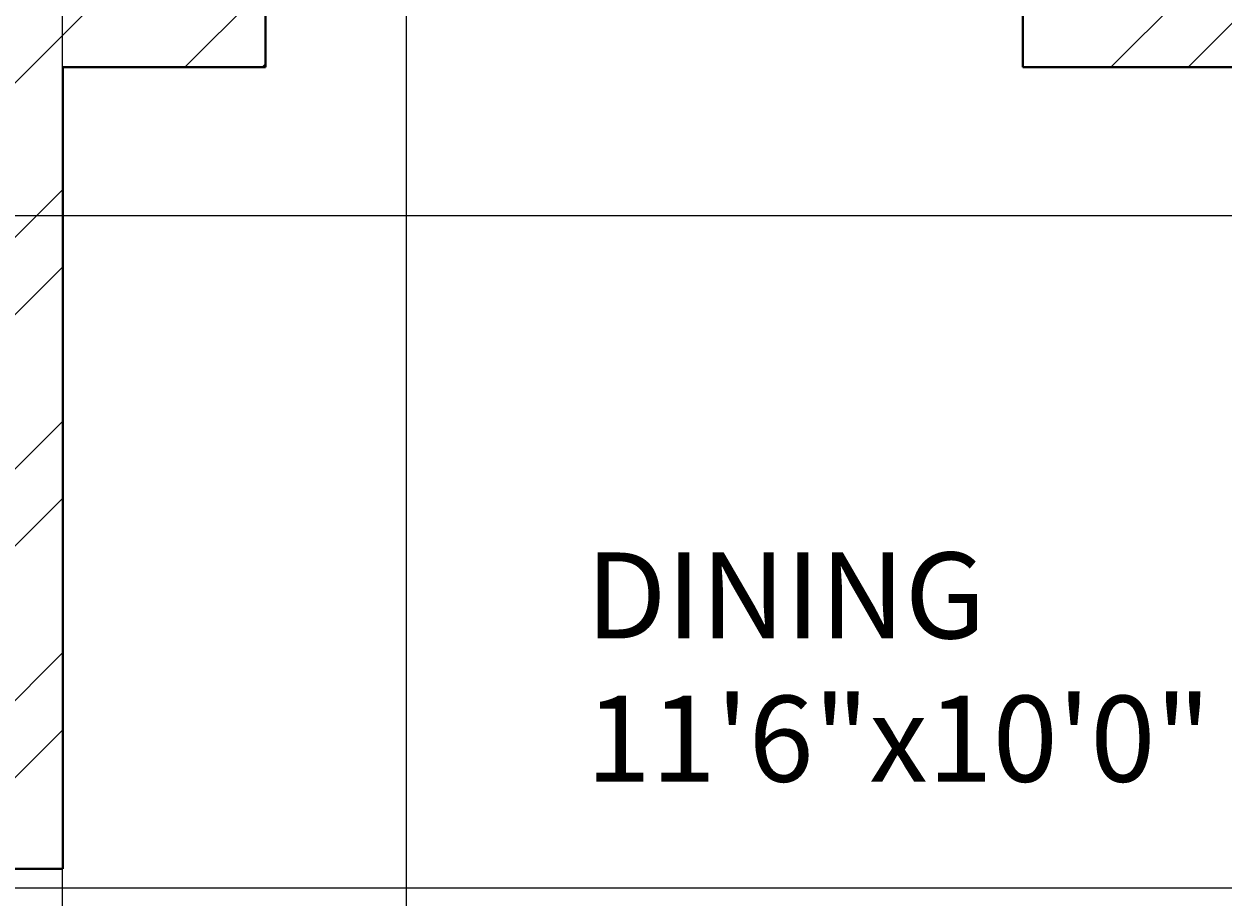
# Model space of a CAD drawing. Units: inches. Extents: x 1601 to 2297, y 1496 to 2631.
# Tile 53 of 57: x 2033 to 2103, y 2371 to 2422. Entities that reach past the tile are written whole.
import ezdxf

# ---------------------------------------------------------------- set-up
doc = ezdxf.new("R2010")
doc.units = ezdxf.units.IN
for name, color, linetype, lineweight in [('A-ANNO-DIMS', 2, 'Continuous', 18), ('A-AREA-IDEN', 7, 'Continuous', 18), ('A-WALL', 7, 'Continuous', 40), ('A-WALL-PATT', 215, 'Continuous', 13)]:
    doc.layers.add(name, color=color, linetype=linetype, lineweight=lineweight)
doc.styles.get("Standard").update_dxf_attribs({"font": 'arial.ttf'})
doc.dimstyles.get("Standard").update_dxf_attribs({"dimtxt": 0.18, "dimasz": 0.18, "dimexe": 0.18, "dimexo": 0.0625, "dimgap": 0.09, "dimtad": 0, "dimtih": 1, "dimtoh": 1, "dimdec": 4, "dimzin": 0, "dimdsep": 46, "dimtxsty": 'Standard', "dimcen": 0.09, "dimadec": 0, "dimazin": 0, "dimtfac": 1, "dimtdec": 4, "dimtofl": 0, "dimtmove": 0, "dimatfit": 3, "dimfxl": 1, "dimtolj": 1, "dimtzin": 0, "dimarcsym": 0})

# ---------------------------------------------------------------- blocks, each defined once
blk = doc.blocks.new('*D40')
at = {"layer": 'A-ANNO-DIMS', "color": 0, "lineweight": -2, "transparency": 16777216}
for p, q in [((2035.537, 1986.388), (2035.537, 2581.055)), ((2035.717, 2580.875), (2045.079, 2580.875)), ((2055.371, 2580.875), (2046.009, 2580.875)), ((2055.551, 1986.388), (2055.551, 2581.055))]:
    blk.add_line(p, q, dxfattribs=at)
at = {"layer": 'A-ANNO-DIMS', "color": 0, "transparency": 16777216}
for points in [[(2035.717, 2580.905), (2035.717, 2580.845), (2035.537, 2580.875)], [(2055.371, 2580.905), (2055.371, 2580.845), (2055.551, 2580.875)]]:
    blk.add_solid(points, dxfattribs=at)
at = {"layer": 'Defpoints', "color": 0, "transparency": 16777216}
for p in [(2055.551, 2580.875), (2035.537, 1986.325), (2055.551, 1986.325)]:
    blk.add_point(p, dxfattribs=at)
at = {"layer": 'A-ANNO-DIMS', "color": 0, "transparency": 16777216, "insert": (2045.544, 2580.875), "char_height": 0.18, "attachment_point": 5}
blk.add_mtext('\\A1;20.014', dxfattribs=at)
blk = doc.blocks.new('*D51')
at = {"layer": 'A-ANNO-DIMS', "color": 0, "lineweight": -2, "transparency": 16777216}
for p, q in [((1912.152, 2411.194), (2279.267, 2411.194)), ((2279.087, 2411.014), (2279.087, 2391.827)), ((2279.087, 2372.275), (2279.087, 2391.463)), ((1912.152, 2372.095), (2279.267, 2372.095))]:
    blk.add_line(p, q, dxfattribs=at)
at = {"layer": 'A-ANNO-DIMS', "color": 0, "transparency": 16777216}
for points in [[(2279.057, 2411.014), (2279.117, 2411.014), (2279.087, 2411.194)], [(2279.057, 2372.275), (2279.117, 2372.275), (2279.087, 2372.095)]]:
    blk.add_solid(points, dxfattribs=at)
at = {"layer": 'Defpoints', "color": 0, "transparency": 16777216}
for p in [(1912.09, 2411.194), (2279.087, 2411.194), (1912.09, 2372.095)]:
    blk.add_point(p, dxfattribs=at)
at = {"layer": 'A-ANNO-DIMS', "color": 0, "transparency": 16777216, "insert": (2279.087, 2391.645), "char_height": 0.18, "attachment_point": 5}
blk.add_mtext('\\A1;39.1', dxfattribs=at)

msp = doc.modelspace()

# ---------------------------------------------------------------- hatches: boundary and pattern name
at = {"layer": 'A-WALL-PATT'}
h = msp.add_hatch(dxfattribs=at)
h.set_pattern_fill('ANSI32', color=256)
h.paths.add_polyline_path([(1842.0336, 2528.0767), (1842.0336, 2532.3254), (1686.0373, 2532.3254), (1686.0373, 2492.9493), (1695.0373, 2492.9493), (1695.0373, 2523.3254), (1827.0373, 2523.3254), (1827.0373, 2416.8254), (1834.6225, 2416.8254), (1834.6225, 2419.0754), (1834.6225, 2421.3254), (1831.5373, 2421.3254), (1831.5373, 2523.3254), (1842.0336, 2523.3254)])
h.paths.add_polyline_path([(1695.0373, 2432.9493), (1686.0373, 2432.9493), (1686.0373, 2325.989), (1695.0373, 2325.989), (1695.0373, 2347.8254), (1827.0373, 2347.8254), (1827.0373, 2287.8254), (1823.2991, 2287.8254), (1823.2991, 2283.3254), (1847.9422, 2283.3254), (1847.9422, 2285.5754), (1847.9422, 2287.8254), (1831.5373, 2287.8254), (1831.5373, 2347.8254), (1846.9946, 2347.8254), (1846.9946, 2350.0754), (1846.9946, 2352.3254), (1695.0373, 2352.3254)])
h.paths.add_polyline_path([(1807.1169, 1573.5395), (2055.0405, 1573.5395), (2055.0405, 1610.6322), (1807.1169, 1610.6322)], flags=9)
h.paths.add_polyline_path([(1841.1631, 1712.7967), (1870.3957, 1712.7967), (1870.3957, 1731.454), (1841.1631, 1731.454)], flags=9)
h.paths.add_polyline_path([(2144.3862, 1772.185), (2191.0233, 1772.185), (2191.0233, 1790.8423), (2144.3862, 1790.8423)], flags=9)
h.paths.add_polyline_path([(2143.0128, 1827.3312), (2177.9958, 1827.3312), (2177.9958, 1845.9886), (2143.0128, 1845.9886)], flags=9)
h.paths.add_polyline_path([(2041.2439, 1833.5691), (2070.8516, 1833.5691), (2070.8516, 1852.2264), (2041.2439, 1852.2264)], flags=9)
h.paths.add_polyline_path([(2097.2791, 1947.0598), (2134.2061, 1947.0598), (2134.2061, 1965.7171), (2097.2791, 1965.7171)], flags=9)
h.paths.add_polyline_path([(2214.995, 1904.3124), (2214.995, 1942.2899), (2196.3376, 1942.2899), (2196.3376, 1904.3124)], flags=9)
h.paths.add_polyline_path([(2186.6284, 2043.8031), (2219.7935, 2043.8031), (2219.7935, 2062.4605), (2186.6284, 2062.4605)], flags=9)
h.paths.add_polyline_path([(2064.0877, 2031.616), (2097.4949, 2031.616), (2097.4949, 2050.2734), (2064.0877, 2050.2734)], flags=9)
h.paths.add_polyline_path([(1973.1349, 1986.0688), (2008.4009, 1986.0688), (2008.4009, 2004.7261), (1973.1349, 2004.7261)], flags=9)
h.paths.add_polyline_path([(1976.3676, 2106.9635), (2005.7469, 2106.9635), (2005.7469, 2125.6209), (1976.3676, 2125.6209)], flags=9)
h.paths.add_polyline_path([(1991.7852, 2180.4863), (2027.0513, 2180.4863), (2027.0513, 2199.1437), (1991.7852, 2199.1437)], flags=9)
h.paths.add_polyline_path([(2106.1801, 2187.9359), (2152.2101, 2187.9359), (2152.2101, 2206.5932), (2106.1801, 2206.5932)], flags=9)
h.paths.add_polyline_path([(2148.6686, 2262.2542), (2182.318, 2262.2542), (2182.318, 2280.9115), (2148.6686, 2280.9115)], flags=9)
h.paths.add_polyline_path([(2041.6327, 2252.8147), (2071.2405, 2252.8147), (2071.2405, 2271.4721), (2041.6327, 2271.4721)], flags=9)
h.paths.add_polyline_path([(2063.9734, 2375.4265), (2100.9004, 2375.4265), (2100.9004, 2394.0839), (2063.9734, 2394.0839)], flags=9)
h.paths.add_polyline_path([(2216.4955, 2330.9748), (2216.4955, 2370.2654), (2197.8381, 2370.2654), (2197.8381, 2330.9748)], flags=9)
h.paths.add_polyline_path([(2179.1416, 2485.8687), (2212.3067, 2485.8687), (2212.3067, 2504.5261), (2179.1416, 2504.5261)], flags=9)
h.paths.add_polyline_path([(2078.7442, 2471.1516), (2112.1514, 2471.1516), (2112.1514, 2489.809), (2078.7442, 2489.809)], flags=9)
h.paths.add_polyline_path([(1915.9631, 2329.4668), (1952.8902, 2329.4668), (1952.8902, 2348.1241), (1915.9631, 2348.1241)], flags=9)
h.paths.add_polyline_path([(1904.3189, 2499.6709), (1940.4512, 2499.6709), (1940.4512, 2518.3282), (1904.3189, 2518.3282)], flags=9)
h.paths.add_polyline_path([(1892.3665, 2100.4595), (1925.6374, 2100.4595), (1925.6374, 2119.1169), (1892.3665, 2119.1169)], flags=9)
h.paths.add_polyline_path([(1909.2984, 1805.9631), (1946.2254, 1805.9631), (1946.2254, 1824.6205), (1909.2984, 1824.6205)], flags=9)
h.paths.add_polyline_path([(1934.6056, 1658.616), (1970.738, 1658.616), (1970.738, 1677.2733), (1934.6056, 1677.2733)], flags=9)
h.paths.add_polyline_path([(1711.2052, 1789.8902), (1750.0456, 1789.8902), (1750.0456, 1808.5476), (1711.2052, 1808.5476)], flags=9)
h.paths.add_polyline_path([(1742.7874, 1854.6743), (1771.9449, 1854.6743), (1771.9449, 1873.3317), (1742.7874, 1873.3317)], flags=9)
h.paths.add_polyline_path([(1807.3592, 1997.7912), (1850.1116, 1997.7912), (1850.1116, 2016.4486), (1807.3592, 2016.4486)], flags=9)
h.paths.add_polyline_path([(1717.4579, 2237.7844), (1760.2103, 2237.7844), (1760.2103, 2256.4417), (1717.4579, 2256.4417)], flags=9)
h.paths.add_polyline_path([(1780.9285, 2324.0623), (1810.086, 2324.0623), (1810.086, 2342.7197), (1780.9285, 2342.7197)], flags=25)
h.paths.add_polyline_path([(1837.696, 2449.2024), (1866.9286, 2449.2024), (1866.9286, 2467.8598), (1837.696, 2467.8598)], flags=9)
h.paths.add_polyline_path([(1712.7752, 2484.9404), (1751.6156, 2484.9404), (1751.6156, 2503.5977), (1712.7752, 2503.5977)], flags=25)
h = msp.add_hatch(dxfattribs=at)
h.set_pattern_fill('ANSI32', color=256)
h.paths.add_polyline_path([(2230.5373, 2532.3254), (2106.0595, 2532.3254), (2106.0595, 2523.3254), (2169.0373, 2523.3254), (2169.0373, 2424.3254), (2091.3989, 2424.3254), (2091.3989, 2419.8254), (2169.0373, 2419.8254), (2169.0373, 2408.1385), (2178.0373, 2408.1385), (2178.0373, 2419.8254), (2181.0581, 2419.8254), (2181.0581, 2422.0754), (2181.0581, 2424.3254), (2178.0373, 2424.3254), (2178.0373, 2523.3254), (2226.0373, 2523.3254), (2226.0373, 2424.3254), (2206.6251, 2424.3254), (2206.6251, 2419.8254), (2226.0373, 2419.8254), (2226.0373, 2299.8254), (2226.0373, 2295.3254), (2178.0373, 2295.3254), (2178.0373, 2312.1385), (2169.0373, 2312.1385), (2169.0373, 2295.3254), (2130.0373, 2295.3254), (2130.0373, 2279.1364), (2128.0593, 2279.1364), (2128.0593, 2274.6364), (2130.0373, 2274.6364), (2130.0373, 2260.7505), (2134.5373, 2260.7505), (2134.5373, 2290.8254), (2226.0373, 2290.8254), (2226.0373, 2279.2475), (2230.5373, 2279.2475), (2230.5373, 2347.8254)])
h.paths.add_polyline_path([(2070.0595, 2532.3254), (2031.0373, 2532.3254), (2031.0373, 2466.3254), (2003.9878, 2466.3254), (2003.9878, 2457.3254), (2031.0373, 2457.3254), (2031.0373, 2419.8254), (2031.0373, 2373.1914), (2035.5373, 2373.1914), (2035.5373, 2419.8254), (2047.3393, 2419.8254), (2047.3393, 2424.3254), (2035.5373, 2424.3254), (2035.5373, 2523.3254), (2070.0595, 2523.3254), (2070.0595, 2527.8254)])
h.paths.add_polyline_path([(1893.0373, 2532.3254), (1866.0336, 2532.3254), (1866.0336, 2523.3254), (1888.5373, 2523.3254), (1888.5373, 2347.8254), (1893.0373, 2347.8254), (1893.0373, 2457.3254), (1907.9878, 2457.3254), (1907.9878, 2466.3254), (1893.0373, 2466.3254)])
h = msp.add_hatch(dxfattribs=at)
h.set_pattern_fill('ANSI32', color=256)
h.paths.add_polyline_path([(1973.9371, 2211.3254), (1893.0373, 2211.3254), (1893.0373, 2287.8254), (1884.6167, 2287.8254), (1884.6167, 2285.5754), (1884.6167, 2283.3254), (1888.5373, 2283.3254), (1888.5373, 2145.3254), (1695.0373, 2145.3254), (1695.0373, 2173.8724), (1690.5373, 2173.8724), (1686.0373, 2173.8724), (1686.0373, 2136.3254), (1722.5687, 2136.3254), (1722.5687, 2117.4352), (1731.5687, 2117.4352), (1731.5687, 2136.3254), (1893.0373, 2136.3254), (1893.0373, 2202.3254), (1959.0373, 2202.3254), (1959.0373, 2182.1303), (1968.0373, 2182.1303), (1968.0373, 2202.3254), (1973.9371, 2202.3254)])
h.paths.add_polyline_path([(2094.0373, 2274.6364), (2096.4294, 2274.6364), (2096.4294, 2276.8864), (2096.4294, 2279.1364), (2094.0373, 2279.1364), (2094.0373, 2290.8254), (2094.0373, 2295.3254), (2089.5373, 2295.3254), (2089.5373, 2230.8254), (2035.5373, 2230.8254), (2035.5373, 2299.8254), (2031.0373, 2299.8254), (2031.0373, 2211.3254), (2023.0065, 2211.3254), (2023.0065, 2202.3254), (2031.0373, 2202.3254), (2031.0373, 2140.8254), (1968.0373, 2140.8254), (1968.0373, 2145.9106), (1963.5373, 2145.9106), (1959.0373, 2145.9106), (1959.0373, 2116.839), (1963.5373, 2116.839), (1968.0373, 2116.839), (1968.0373, 2131.8254), (2031.0373, 2131.8254), (2031.0373, 2094.3254), (2031.0373, 2085.3254), (2031.0373, 2056.8254), (1968.0373, 2056.8254), (1968.0373, 2070.4947), (1963.5373, 2070.4947), (1959.0373, 2070.4947), (1959.0373, 2040.3029), (1968.0373, 2040.3029), (1968.0373, 2047.8254), (2031.0373, 2047.8254), (2031.0373, 1983.3254), (2031.0373, 1978.8254), (2021.1979, 1978.8254), (2021.1979, 1974.3254), (2031.0373, 1974.3254), (2031.0373, 1954.3528), (2035.5373, 1954.3528), (2035.5373, 1974.3254), (2035.5373, 1981.8254), (2055.5513, 1981.8254), (2055.5513, 1986.3254), (2035.5373, 1986.3254), (2035.5373, 2047.8254), (2040.0373, 2047.8254), (2040.0373, 2085.3254), (2040.0373, 2094.3254), (2040.0373, 2140.8254), (2035.5373, 2140.8254), (2035.5373, 2226.3254), (2089.5373, 2226.3254), (2094.0373, 2226.3254)])
h.paths.add_polyline_path([(2226.0373, 2230.8254), (2134.5373, 2230.8254), (2134.5373, 2233.5437), (2130.0373, 2233.5437), (2130.0373, 2226.3254), (2134.5373, 2226.3254), (2226.0373, 2226.3254)])
h.paths.add_polyline_path([(1807.1169, 1573.5395), (2055.0405, 1573.5395), (2055.0405, 1610.6322), (1807.1169, 1610.6322)], flags=9)
h.paths.add_polyline_path([(1841.1631, 1712.7967), (1870.3957, 1712.7967), (1870.3957, 1731.454), (1841.1631, 1731.454)], flags=9)
h.paths.add_polyline_path([(2144.3862, 1772.185), (2191.0233, 1772.185), (2191.0233, 1790.8423), (2144.3862, 1790.8423)], flags=9)
h.paths.add_polyline_path([(2143.0128, 1827.3312), (2177.9958, 1827.3312), (2177.9958, 1845.9886), (2143.0128, 1845.9886)], flags=9)
h.paths.add_polyline_path([(2041.2439, 1833.5691), (2070.8516, 1833.5691), (2070.8516, 1852.2264), (2041.2439, 1852.2264)], flags=9)
h.paths.add_polyline_path([(2097.2791, 1947.0598), (2134.2061, 1947.0598), (2134.2061, 1965.7171), (2097.2791, 1965.7171)], flags=9)
h.paths.add_polyline_path([(2214.995, 1904.3124), (2214.995, 1942.2899), (2196.3376, 1942.2899), (2196.3376, 1904.3124)], flags=9)
h.paths.add_polyline_path([(2186.6284, 2043.8031), (2219.7935, 2043.8031), (2219.7935, 2062.4605), (2186.6284, 2062.4605)], flags=9)
h.paths.add_polyline_path([(2064.0877, 2031.616), (2097.4949, 2031.616), (2097.4949, 2050.2734), (2064.0877, 2050.2734)], flags=9)
h.paths.add_polyline_path([(1973.1349, 1986.0688), (2008.4009, 1986.0688), (2008.4009, 2004.7261), (1973.1349, 2004.7261)], flags=25)
h.paths.add_polyline_path([(1976.3676, 2106.9635), (2005.7469, 2106.9635), (2005.7469, 2125.6209), (1976.3676, 2125.6209)], flags=25)
h.paths.add_polyline_path([(1991.7852, 2180.4863), (2027.0513, 2180.4863), (2027.0513, 2199.1437), (1991.7852, 2199.1437)], flags=25)
h.paths.add_polyline_path([(2106.1801, 2187.9359), (2152.2101, 2187.9359), (2152.2101, 2206.5932), (2106.1801, 2206.5932)], flags=9)
h.paths.add_polyline_path([(2148.6686, 2262.2542), (2182.318, 2262.2542), (2182.318, 2280.9115), (2148.6686, 2280.9115)], flags=9)
h.paths.add_polyline_path([(2041.6327, 2252.8147), (2071.2405, 2252.8147), (2071.2405, 2271.4721), (2041.6327, 2271.4721)], flags=25)
h.paths.add_polyline_path([(2063.9734, 2375.4265), (2100.9004, 2375.4265), (2100.9004, 2394.0839), (2063.9734, 2394.0839)], flags=9)
h.paths.add_polyline_path([(2216.4955, 2330.9748), (2216.4955, 2370.2654), (2197.8381, 2370.2654), (2197.8381, 2330.9748)], flags=9)
h.paths.add_polyline_path([(2179.1416, 2485.8687), (2212.3067, 2485.8687), (2212.3067, 2504.5261), (2179.1416, 2504.5261)], flags=9)
h.paths.add_polyline_path([(2078.7442, 2471.1516), (2112.1514, 2471.1516), (2112.1514, 2489.809), (2078.7442, 2489.809)], flags=9)
h.paths.add_polyline_path([(1915.9631, 2329.4668), (1952.8902, 2329.4668), (1952.8902, 2348.1241), (1915.9631, 2348.1241)], flags=9)
h.paths.add_polyline_path([(1904.3189, 2499.6709), (1940.4512, 2499.6709), (1940.4512, 2518.3282), (1904.3189, 2518.3282)], flags=9)
h.paths.add_polyline_path([(1892.3665, 2100.4595), (1925.6374, 2100.4595), (1925.6374, 2119.1169), (1892.3665, 2119.1169)], flags=9)
h.paths.add_polyline_path([(1909.2984, 1805.9631), (1946.2254, 1805.9631), (1946.2254, 1824.6205), (1909.2984, 1824.6205)], flags=9)
h.paths.add_polyline_path([(1934.6056, 1658.616), (1970.738, 1658.616), (1970.738, 1677.2733), (1934.6056, 1677.2733)], flags=9)
h.paths.add_polyline_path([(1711.2052, 1789.8902), (1750.0456, 1789.8902), (1750.0456, 1808.5476), (1711.2052, 1808.5476)], flags=9)
h.paths.add_polyline_path([(1742.7874, 1854.6743), (1771.9449, 1854.6743), (1771.9449, 1873.3317), (1742.7874, 1873.3317)], flags=9)
h.paths.add_polyline_path([(1807.3592, 1997.7912), (1850.1116, 1997.7912), (1850.1116, 2016.4486), (1807.3592, 2016.4486)], flags=9)
h.paths.add_polyline_path([(1717.4579, 2237.7844), (1760.2103, 2237.7844), (1760.2103, 2256.4417), (1717.4579, 2256.4417)], flags=25)
h.paths.add_polyline_path([(1780.9285, 2324.0623), (1810.086, 2324.0623), (1810.086, 2342.7197), (1780.9285, 2342.7197)], flags=9)
h.paths.add_polyline_path([(1837.696, 2449.2024), (1866.9286, 2449.2024), (1866.9286, 2467.8598), (1837.696, 2467.8598)], flags=9)
h.paths.add_polyline_path([(1712.7752, 2484.9404), (1751.6156, 2484.9404), (1751.6156, 2503.5977), (1712.7752, 2503.5977)], flags=9)
h = msp.add_hatch(dxfattribs=at)
h.set_pattern_fill('ANSI32', color=256)
h.paths.add_polyline_path([(2230.5373, 1861.8254), (2182.5373, 1861.8254), (2182.5373, 1885.3637), (2178.0373, 1885.3637), (2178.0373, 1861.8254), (2166.0373, 1861.8254), (2134.5373, 1861.8254), (2130.0373, 1861.8254), (2130.0373, 1841.4682), (2126.8833, 1841.4682), (2126.8833, 1836.9682), (2130.0373, 1836.9682), (2130.0373, 1822.7302), (2134.5373, 1822.7302), (2134.5373, 1857.3254), (2166.0373, 1857.3254), (2226.0373, 1857.3254), (2226.0373, 1846.1155), (2230.5373, 1846.1155)])
h.paths.add_polyline_path([(2226.0373, 1797.3254), (2134.5373, 1797.3254), (2134.5373, 1800.6636), (2132.2873, 1800.6636), (2130.0373, 1800.6636), (2130.0373, 1797.3254), (2130.0373, 1792.8254), (2167.7264, 1792.8254), (2226.0373, 1792.8254)])
h.paths.add_polyline_path([(2230.5373, 1822.1155), (2226.0373, 1822.1155), (2226.0373, 1760.8563), (2230.5373, 1760.8563)])
h.paths.add_polyline_path([(2230.5373, 1700.8563), (2226.0373, 1700.8563), (2226.0373, 1644.3254), (2140.2517, 1644.3254), (2140.2517, 1635.3254), (2230.5373, 1635.3254)])
h.paths.add_polyline_path([(2080.2517, 1639.8254), (2080.2517, 1644.3254), (2035.5373, 1644.3254), (2035.5373, 1792.8254), (2094.0373, 1792.8254), (2094.0373, 1797.3254), (2094.0373, 1836.9682), (2097.1057, 1836.9682), (2097.1057, 1839.2182), (2097.1057, 1841.4682), (2094.0373, 1841.4682), (2094.0373, 1862.2276), (2089.5373, 1862.2276), (2089.5373, 1797.3254), (2035.5373, 1797.3254), (2035.5373, 1857.3254), (2035.5373, 1885.0916), (2031.0373, 1885.0916), (2031.0373, 1710.3254), (2012.329, 1710.3254), (2012.329, 1701.3254), (2031.0373, 1701.3254), (2031.0373, 1644.3254), (2031.0373, 1635.3254), (2080.2517, 1635.3254)])
h.paths.add_polyline_path([(1836.0373, 1653.2033), (1842.6171, 1653.2033), (1842.6171, 1657.7033), (1842.6171, 1662.2033), (1831.5373, 1662.2033), (1831.5373, 1764.2033), (1835.3881, 1764.2033), (1835.3881, 1766.4533), (1835.3881, 1768.7033), (1831.5373, 1768.7033), (1827.0373, 1768.7033), (1827.0373, 1662.2033), (1827.0373, 1635.3254), (1836.0373, 1635.3254)])
h.paths.add_polyline_path([(1893.0373, 1701.3254), (1907.193, 1701.3254), (1907.193, 1705.8254), (1907.193, 1710.3254), (1893.0373, 1710.3254), (1893.0373, 1819.8254), (1882.6444, 1819.8254), (1882.6444, 1817.5754), (1882.6444, 1815.3254), (1888.5373, 1815.3254), (1888.5373, 1662.2033), (1884.0373, 1662.2033), (1866.6171, 1662.2033), (1866.6171, 1653.2033), (1882.391, 1653.2033), (1884.0373, 1653.2033), (1884.0373, 1635.3254), (1893.0373, 1635.3254)])
h.paths.add_polyline_path([(1739.3335, 1639.8254), (1739.3335, 1644.3254), (1695.0373, 1644.3254), (1695.0373, 1702.0135), (1690.5373, 1702.0135), (1686.0373, 1702.0135), (1686.0373, 1635.3254), (1739.3335, 1635.3254)])
h.paths.add_polyline_path([(1827.0373, 1644.3254), (1799.3335, 1644.3254), (1799.3335, 1635.3254), (1827.0373, 1635.3254)])
h.paths.add_polyline_path([(1695.0373, 1815.3254), (1849.2759, 1815.3254), (1849.2759, 1819.8254), (1807.5373, 1819.8254), (1807.5373, 1879.8254), (1851.1533, 1879.8254), (1851.1533, 1882.0754), (1851.1533, 1884.3254), (1799.3405, 1884.3254), (1799.3405, 1882.0754), (1799.3405, 1879.8254), (1803.0373, 1879.8254), (1803.0373, 1819.8254), (1695.0373, 1819.8254), (1695.0373, 1835.0458), (1690.5373, 1835.0458), (1686.0373, 1835.0458), (1686.0373, 1766.1753), (1695.0373, 1766.1753)])
h.paths.add_polyline_path([(1775.8157, 1884.3254), (1695.0373, 1884.3254), (1695.0373, 1912.9526), (1690.5373, 1912.9526), (1686.0373, 1912.9526), (1686.0373, 1859.0458), (1695.0373, 1859.0458), (1695.0373, 1879.8254), (1775.8157, 1879.8254)])
h.paths.add_polyline_path([(1893.0373, 2031.3254), (1731.5687, 2031.3254), (1731.5687, 2057.4352), (1722.5687, 2057.4352), (1722.5687, 2031.3254), (1686.0373, 2031.3254), (1686.0373, 1972.9526), (1695.0373, 1972.9526), (1695.0373, 2022.3254), (1888.5373, 2022.3254), (1888.5373, 1884.3254), (1883.4996, 1884.3254), (1883.4996, 1879.8254), (1893.0373, 1879.8254), (1893.0373, 1974.3254), (1976.6199, 1974.3254), (1976.6199, 1978.8254), (1968.0373, 1978.8254), (1968.0373, 1983.3254), (1968.0373, 2008.4756), (1963.5373, 2008.4756), (1959.0373, 2008.4756), (1959.0373, 1983.3254), (1893.0373, 1983.3254)])
h.paths.add_polyline_path([(2230.5373, 2140.4745), (2226.0373, 2140.4745), (2226.0373, 2094.3254), (2040.0373, 2094.3254), (2040.0373, 2085.3254), (2178.0373, 2085.3254), (2178.0373, 2065.6965), (2182.5373, 2065.6965), (2182.5373, 2085.3254), (2226.0373, 2085.3254), (2226.0373, 1986.3254), (2211.2679, 1986.3254), (2211.2679, 1981.8254), (2230.5373, 1981.8254)])
h.paths.add_polyline_path([(2187.6292, 1986.3254), (2182.5373, 1986.3254), (2182.5373, 2029.6965), (2178.0373, 2029.6965), (2178.0373, 1986.3254), (2099.05, 1986.3254), (2099.05, 1981.8254), (2178.0373, 1981.8254), (2178.0373, 1969.3637), (2182.5373, 1969.3637), (2182.5373, 1981.8254), (2187.6292, 1981.8254), (2187.6292, 1984.0754)])
h.paths.add_polyline_path([(1807.1169, 1573.5395), (2055.0405, 1573.5395), (2055.0405, 1610.6322), (1807.1169, 1610.6322)], flags=9)
h.paths.add_polyline_path([(1841.1631, 1712.7967), (1870.3957, 1712.7967), (1870.3957, 1731.454), (1841.1631, 1731.454)], flags=9)
h.paths.add_polyline_path([(2144.3862, 1772.185), (2191.0233, 1772.185), (2191.0233, 1790.8423), (2144.3862, 1790.8423)], flags=9)
h.paths.add_polyline_path([(2143.0128, 1827.3312), (2177.9958, 1827.3312), (2177.9958, 1845.9886), (2143.0128, 1845.9886)], flags=25)
h.paths.add_polyline_path([(2041.2439, 1833.5691), (2070.8516, 1833.5691), (2070.8516, 1852.2264), (2041.2439, 1852.2264)], flags=25)
h.paths.add_polyline_path([(2097.2791, 1947.0598), (2134.2061, 1947.0598), (2134.2061, 1965.7171), (2097.2791, 1965.7171)], flags=9)
h.paths.add_polyline_path([(2214.995, 1904.3124), (2214.995, 1942.2899), (2196.3376, 1942.2899), (2196.3376, 1904.3124)], flags=9)
h.paths.add_polyline_path([(2186.6284, 2043.8031), (2219.7935, 2043.8031), (2219.7935, 2062.4605), (2186.6284, 2062.4605)], flags=25)
h.paths.add_polyline_path([(2064.0877, 2031.616), (2097.4949, 2031.616), (2097.4949, 2050.2734), (2064.0877, 2050.2734)], flags=25)
h.paths.add_polyline_path([(1973.1349, 1986.0688), (2008.4009, 1986.0688), (2008.4009, 2004.7261), (1973.1349, 2004.7261)], flags=9)
h.paths.add_polyline_path([(1976.3676, 2106.9635), (2005.7469, 2106.9635), (2005.7469, 2125.6209), (1976.3676, 2125.6209)], flags=9)
h.paths.add_polyline_path([(1991.7852, 2180.4863), (2027.0513, 2180.4863), (2027.0513, 2199.1437), (1991.7852, 2199.1437)], flags=9)
h.paths.add_polyline_path([(2106.1801, 2187.9359), (2152.2101, 2187.9359), (2152.2101, 2206.5932), (2106.1801, 2206.5932)], flags=9)
h.paths.add_polyline_path([(2148.6686, 2262.2542), (2182.318, 2262.2542), (2182.318, 2280.9115), (2148.6686, 2280.9115)], flags=9)
h.paths.add_polyline_path([(2041.6327, 2252.8147), (2071.2405, 2252.8147), (2071.2405, 2271.4721), (2041.6327, 2271.4721)], flags=9)
h.paths.add_polyline_path([(2063.9734, 2375.4265), (2100.9004, 2375.4265), (2100.9004, 2394.0839), (2063.9734, 2394.0839)], flags=9)
h.paths.add_polyline_path([(2216.4955, 2330.9748), (2216.4955, 2370.2654), (2197.8381, 2370.2654), (2197.8381, 2330.9748)], flags=9)
h.paths.add_polyline_path([(2179.1416, 2485.8687), (2212.3067, 2485.8687), (2212.3067, 2504.5261), (2179.1416, 2504.5261)], flags=9)
h.paths.add_polyline_path([(2078.7442, 2471.1516), (2112.1514, 2471.1516), (2112.1514, 2489.809), (2078.7442, 2489.809)], flags=9)
h.paths.add_polyline_path([(1915.9631, 2329.4668), (1952.8902, 2329.4668), (1952.8902, 2348.1241), (1915.9631, 2348.1241)], flags=9)
h.paths.add_polyline_path([(1904.3189, 2499.6709), (1940.4512, 2499.6709), (1940.4512, 2518.3282), (1904.3189, 2518.3282)], flags=9)
h.paths.add_polyline_path([(1892.3665, 2100.4595), (1925.6374, 2100.4595), (1925.6374, 2119.1169), (1892.3665, 2119.1169)], flags=9)
h.paths.add_polyline_path([(1909.2984, 1805.9631), (1946.2254, 1805.9631), (1946.2254, 1824.6205), (1909.2984, 1824.6205)], flags=9)
h.paths.add_polyline_path([(1934.6056, 1658.616), (1970.738, 1658.616), (1970.738, 1677.2733), (1934.6056, 1677.2733)], flags=9)
h.paths.add_polyline_path([(1711.2052, 1789.8902), (1750.0456, 1789.8902), (1750.0456, 1808.5476), (1711.2052, 1808.5476)], flags=25)
h.paths.add_polyline_path([(1742.7874, 1854.6743), (1771.9449, 1854.6743), (1771.9449, 1873.3317), (1742.7874, 1873.3317)], flags=25)
h.paths.add_polyline_path([(1807.3592, 1997.7912), (1850.1116, 1997.7912), (1850.1116, 2016.4486), (1807.3592, 2016.4486)], flags=25)
h.paths.add_polyline_path([(1717.4579, 2237.7844), (1760.2103, 2237.7844), (1760.2103, 2256.4417), (1717.4579, 2256.4417)], flags=9)
h.paths.add_polyline_path([(1780.9285, 2324.0623), (1810.086, 2324.0623), (1810.086, 2342.7197), (1780.9285, 2342.7197)], flags=9)
h.paths.add_polyline_path([(1837.696, 2449.2024), (1866.9286, 2449.2024), (1866.9286, 2467.8598), (1837.696, 2467.8598)], flags=9)
h.paths.add_polyline_path([(1712.7752, 2484.9404), (1751.6156, 2484.9404), (1751.6156, 2503.5977), (1712.7752, 2503.5977)], flags=9)

# ---------------------------------------------------------------- linework, layer by layer
at = {"layer": 'A-WALL'}
for p, q in [((2047.3393, 2424.3254), (2047.3393, 2419.8254)), ((2091.3989, 2424.3254), (2091.3989, 2419.8254)), ((2035.5373, 2419.8254), (2047.3393, 2419.8254)), ((2035.5373, 2373.1914), (2035.5373, 2419.8254)), ((2091.3989, 2419.8254), (2169.0373, 2419.8254)), ((2031.0373, 2373.1914), (2035.5373, 2373.1914))]:
    msp.add_line(p, q, dxfattribs=at)

# ---------------------------------------------------------------- texts
at = {"layer": 'A-AREA-IDEN', "insert": (2065.984, 2391.5958), "char_height": 5, "attachment_point": 1}
msp.add_mtext_dynamic_manual_height_columns('DINING\\P11\'6"x10\'0"', width=68.737134, gutter_width=12.5, heights=[0], dxfattribs=at)

# ---------------------------------------------------------------- dimensions: what is measured, and where the dimension line sits
at = {"layer": 'A-ANNO-DIMS'}
dim = msp.add_linear_dim(base=(2055.5513, 2580.8754), p1=(2035.5373, 1986.3254), p2=(2055.5513, 1986.3254), dimstyle='Standard', override={"dimdec": 3, "dimlfac": 1, "dimrnd": 0, "dimzin": 0, "dimdsep": 46, "dimlunit": 2}, dxfattribs=at)
dim.commit()
dim.dimension.update_dxf_attribs({"geometry": '*D40', "text_midpoint": (2045.5443, 2580.8754)})
dim = msp.add_linear_dim(base=(2279.0873, 2411.1939), p1=(1912.0896, 2372.0953), p2=(1912.0896, 2411.1939), angle=90, dimstyle='Standard', override={"dimdec": 1, "dimlfac": 1, "dimrnd": 0, "dimzin": 0, "dimdsep": 46, "dimlunit": 2}, dxfattribs=at)
dim.commit()
dim.dimension.update_dxf_attribs({"geometry": '*D51', "text_midpoint": (2279.0873, 2391.6446)})

doc.saveas('drawing.dxf')
